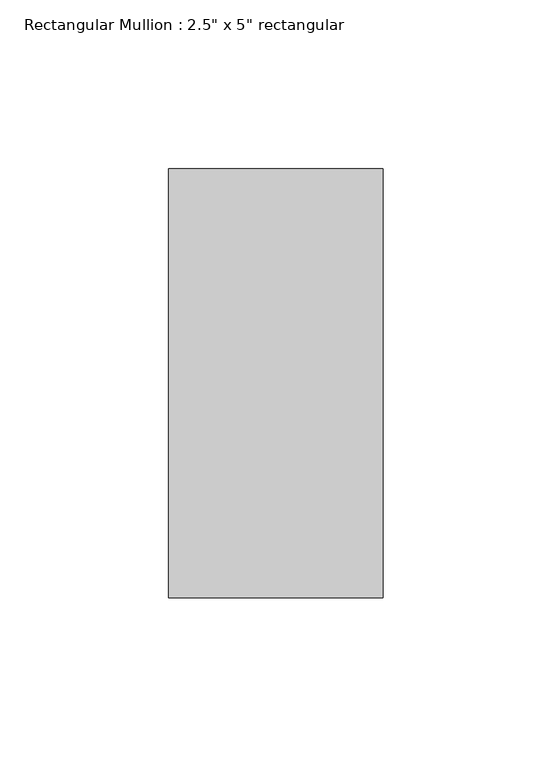
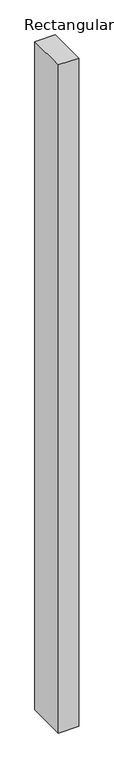
"""IFC4 building model written with IfcOpenShell, lengths in millimetres: member geometry."""

from ifc_helpers import new_model, si_unit, frame, origin, place, context, project, spatial, polyline, outline, extrude, source, transform, mapped, element, save


def member_76111e69(model_context):
    return source(origin(), model_context, "Body", "SweptSolid", [
        extrude(outline(polyline([(0.0, 63.5), (0.0, -63.5), (-63.5, -63.5), (-63.5, 63.5), (0.0, 63.5)])), frame((0.0, 0.0, -2209.8), z_axis=(0.0, 0.0, 1.0), x_axis=(1.0, 0.0, 0.0)), (0.0, 0.0, 1.0), 2209.8),
    ])


if __name__ == "__main__":
    model = new_model("IFC4")
    model_context = context("Model", 3, world=origin())
    ifc_project = project(units=[si_unit("LENGTHUNIT", "METRE", prefix="MILLI")], contexts=[model_context])
    site = spatial("IfcSite", under=ifc_project)
    building = spatial("IfcBuilding", under=site)
    placement = place(None, origin())
    member_shape = member_76111e69(model_context)
    element("IfcMember", 1, ObjectType="Rectangular Mullion : 2.5\" x 5\" rectangular", at=placement, inside=building, context=model_context, shape_type="MappedRepresentation", body=[
        mapped(member_shape, transform((0.0, 0.0, 0.0), x_axis=(1.0, 0.0, 0.0), y_axis=(0.0, 1.0, 0.0), z_axis=(0.0, 0.0, 1.0))),
    ])
    save(model, "model.ifc")

# Revit data of these elements
# Type "Rectangular Mullion : 2.5\" x 5\" rectangular"
#   built-in parameter 1007304 = 0.416667 (stored number, unit not read)
#   built-in parameter 1007301 = 0.104167 (stored number, unit not read)
#   built-in parameter 1007300 = 0.104167 (stored number, unit not read)
# Element 1 (IfcMember, "Rectangular Mullion : 2.5\" x 5\" rectangular")
#   Materials on its faces: "Aluminum"
# Materials
#   "Aluminum": class "Metal", colour RGB 247 247 247, transparency 0, Description = "Aluminum 6061", Cost = 0
